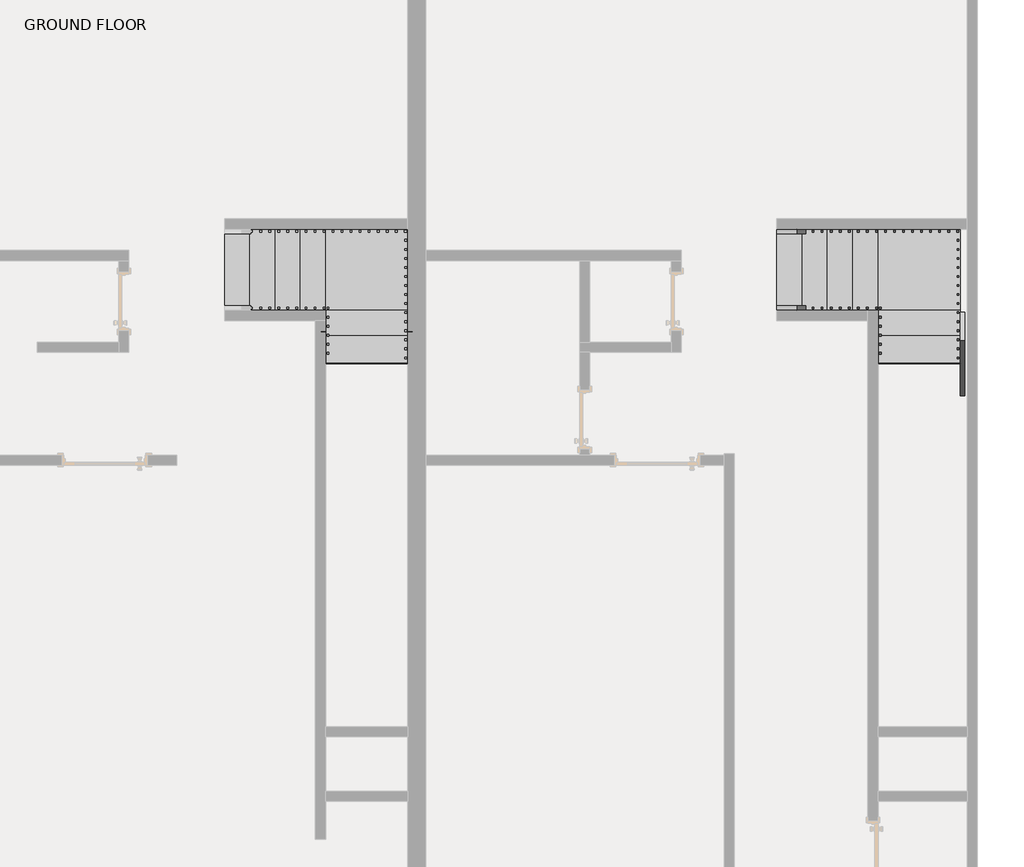
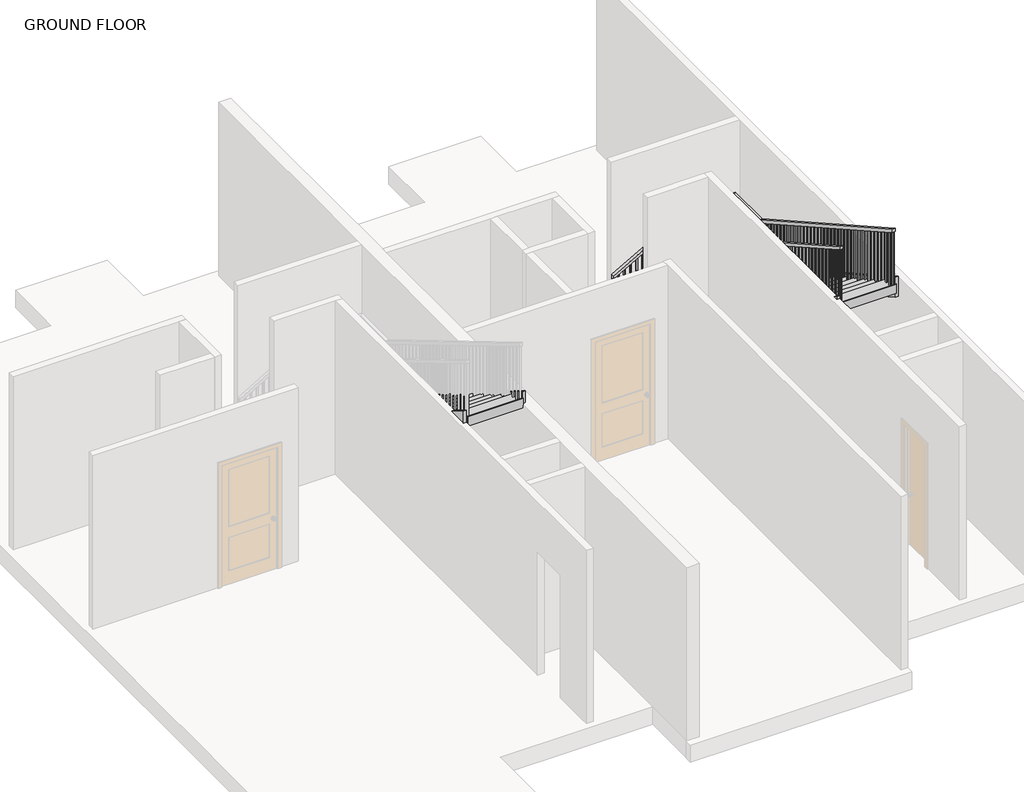
# One storey, part 4 of 4: 8 members, 2 railings, 2 stair flights.
"""IFC4 building model written with IfcOpenShell, lengths in millimetres."""

from ifc_helpers import new_model, si_unit, frame, origin, place, context, project, spatial, polyline, outline, extrude, faceted_brep, transform, mapped, element, save
from components import stair_flight_9587ce78, stair_flight_92322d8c

model = new_model("IFC4")

# Units and contexts
model_context = context("Model", 3, world=origin())
ifc_project = project(units=[si_unit("LENGTHUNIT", "METRE", prefix="MILLI")], contexts=[model_context])

# Site, building, storey
site = spatial("IfcSite", under=ifc_project)
building = spatial("IfcBuilding", under=site)
storey = spatial("IfcBuildingStorey", under=building, Name="GROUND FLOOR", Elevation=304.8)

# Members
placement = place(None, origin())
element("IfcMember", 1, ObjectType="Stringer - 2\" Width", at=placement, inside=storey, context=model_context, shape_type="SweptSolid", body=[
    extrude(outline(polyline([(516.0200704, -14204.9595293), (304.8, -14204.9595293), (304.8, -13964.03282), (818.2858896, -13102.7637874), (818.2858896, -13697.9695712), (516.0200704, -14204.9595293)])), frame((0.0, 4044.5909199, 0.0), z_axis=(0.0, 1.0, 0.0), x_axis=(0.0, 0.0, 1.0)), (0.0, 0.0, 1.0), 50.8),
])
element("IfcMember", 2, ObjectType="Stringer - 2\" Width", at=placement, inside=storey, context=model_context, shape_type="SweptSolid", body=[
    extrude(outline(polyline([(2488.0796213, 1390.0849918), (-567.9697052, 3209.1936945), (-567.9697052, 3563.90557), (3083.9851801, 1390.0849918), (2488.0796213, 1390.0849918)])), frame((-12143.6860997, 0.0, 0.0), z_axis=(1.0, 0.0, 0.0), x_axis=(0.0, 1.0, 0.0)), (0.0, 0.0, 1.0), 50.8),
])
element("IfcMember", 3, ObjectType="Stringer - 2\" Width", at=placement, inside=storey, context=model_context, shape_type="SweptSolid", body=[
    extrude(outline(polyline([(516.0200704, -14204.9595293), (304.8, -14204.9595293), (304.8, -13964.03282), (808.1881543, -13119.7007021), (1163.0479714, -13119.7007021), (516.0200704, -14204.9595293)])), frame((0.0, 3079.3909199, 0.0), z_axis=(0.0, 1.0, 0.0), x_axis=(0.0, 0.0, 1.0)), (0.0, 0.0, 1.0), 50.8),
])
element("IfcMember", 4, ObjectType="Stringer - 2\" Width", at=placement, inside=storey, context=model_context, shape_type="SweptSolid", body=[
    extrude(outline(polyline([(3130.1909199, 1362.5810956), (3130.1909199, 1007.8692202), (-567.9697052, 3209.1936945), (-567.9697052, 3563.90557), (3130.1909199, 1362.5810956)])), frame((-13119.7007021, 0.0, 0.0), z_axis=(1.0, 0.0, 0.0), x_axis=(0.0, 1.0, 0.0)), (0.0, 0.0, 1.0), 50.8),
])
element("IfcMember", 5, ObjectType="Stringer - 2\" Width", at=placement, inside=storey, context=model_context, shape_type="SweptSolid", body=[
    extrude(outline(polyline([(513.2142827, -7996.544927), (304.8, -7996.544927), (304.8, -7745.7665395), (799.5757743, -6869.775142), (799.5757743, -7489.5471791), (513.2142827, -7996.544927)])), frame((0.0, 4044.5909199, 0.0), z_axis=(0.0, 1.0, 0.0), x_axis=(0.0, 0.0, 1.0)), (0.0, 0.0, 1.0), 50.8),
])
element("IfcMember", 6, ObjectType="Stringer - 2\" Width", at=placement, inside=storey, context=model_context, shape_type="SweptSolid", body=[
    extrude(outline(polyline([(2488.0775681, 1327.4003232), (-567.9697052, 3050.7653048), (-567.9697052, 3400.6891557), (3108.5983757, 1327.4003232), (2488.0775681, 1327.4003232)])), frame((-5935.2714974, 0.0, 0.0), z_axis=(1.0, 0.0, 0.0), x_axis=(0.0, 1.0, 0.0)), (0.0, 0.0, 1.0), 50.8),
])
element("IfcMember", 7, ObjectType="Stringer - 2\" Width", at=placement, inside=storey, context=model_context, shape_type="SweptSolid", body=[
    extrude(outline(polyline([(513.2142827, -7996.544927), (304.8, -7996.544927), (304.8, -7745.7665395), (776.1296351, -6911.2860997), (1126.1880836, -6911.2860997), (513.2142827, -7996.544927)])), frame((0.0, 3079.3909199, 0.0), z_axis=(0.0, 1.0, 0.0), x_axis=(0.0, 0.0, 1.0)), (0.0, 0.0, 1.0), 50.8),
])
element("IfcMember", 8, ObjectType="Stringer - 2\" Width", at=placement, inside=storey, context=model_context, shape_type="SweptSolid", body=[
    extrude(outline(polyline([(3130.1909199, 1315.2238642), (3130.1909199, 965.3000133), (-567.9697052, 3050.7653048), (-567.9697052, 3400.6891557), (3130.1909199, 1315.2238642)])), frame((-6911.2860997, 0.0, 0.0), z_axis=(1.0, 0.0, 0.0), x_axis=(0.0, 1.0, 0.0)), (0.0, 0.0, 1.0), 50.8),
])

# Railings
element("IfcRailing", 9, ObjectType="Handrail - Rectangular", at=placement, inside=storey, context=model_context, shape_type="SolidModel", body=[
    faceted_brep([(-7996.544927, 3180.9909199, 1379.6210526), (-7996.544927, 3180.9909199, 1321.2775897), (-7996.544927, 3130.1909199, 1321.2775897), (-7996.544927, 3130.1909199, 1379.6210526), (-6936.6860997, 3180.9909199, 1978.2649419), (-6885.8860997, 3180.9909199, 1948.6150265), (-6885.8860997, 3130.1909199, 1948.6150265), (-6936.6860997, 3130.1909199, 1978.2649419), (-6936.6860997, 3180.9909199, 2224.6971629), (-6885.8860997, 3180.9909199, 2173.8971629), (-6885.8860997, 3130.1909199, 2173.8971629), (-6936.6860997, 3130.1909199, 2224.6971629), (-6809.6860997, 3180.9909199, 2224.6971629), (-6809.6860997, 3180.9909199, 2173.8971629), (-6860.4860997, 3130.1909199, 2173.8971629), (-6860.4860997, 3130.1909199, 2224.6971629), (-6809.6860997, 3053.9909199, 2224.6971629), (-6809.6860997, 3040.6545009, 2173.8971629), (-6860.4860997, 3040.6545009, 2173.8971629), (-6860.4860997, 3053.9909199, 2224.6971629), (-6809.6860997, -567.9697052, 4267.2), (-6860.4860997, -567.9697052, 4267.2), (-6860.4860997, -567.9697052, 4208.8793016), (-6809.6860997, -567.9697052, 4208.8793016)], [[[0, 1, 2, 3]], [[1, 0, 4, 5]], [[2, 1, 5, 6]], [[3, 2, 6, 7]], [[0, 3, 7, 4]], [[5, 4, 8, 9]], [[6, 5, 9, 10]], [[7, 6, 10, 11]], [[4, 7, 11, 8]], [[9, 8, 12, 13]], [[10, 9, 13, 14]], [[11, 10, 14, 15]], [[8, 11, 15, 12]], [[13, 12, 16, 17]], [[14, 13, 17, 18]], [[15, 14, 18, 19]], [[12, 15, 19, 16]], [[20, 21, 22, 23]], [[17, 16, 20, 23]], [[18, 17, 23, 22]], [[19, 18, 22, 21]], [[16, 19, 21, 20]]]),
    extrude(outline(polyline([(-511.5340801, 4177.0195862), (-492.4840801, 4166.2768744), (-492.4840801, 3192.3789474), (-511.5340801, 3192.3789474), (-511.5340801, 4177.0195862)])), frame((-6844.6110997, 0.0, 0.0), z_axis=(1.0, 0.0, 0.0), x_axis=(0.0, 1.0, 0.0)), (0.0, 0.0, 1.0), 19.05),
    extrude(outline(polyline([(-409.9340801, 4119.7251234), (-390.8840801, 4108.9824116), (-390.8840801, 3192.3789474), (-409.9340801, 3192.3789474), (-409.9340801, 4119.7251234)])), frame((-6844.6110997, 0.0, 0.0), z_axis=(1.0, 0.0, 0.0), x_axis=(0.0, 1.0, 0.0)), (0.0, 0.0, 1.0), 19.05),
    extrude(outline(polyline([(-308.3340801, 4062.4306606), (-289.2840801, 4051.6879488), (-289.2840801, 3192.3789474), (-308.3340801, 3192.3789474), (-308.3340801, 4062.4306606)])), frame((-6844.6110997, 0.0, 0.0), z_axis=(1.0, 0.0, 0.0), x_axis=(0.0, 1.0, 0.0)), (0.0, 0.0, 1.0), 19.05),
    extrude(outline(polyline([(-206.7340801, 4005.1361978), (-187.6840801, 3994.393486), (-187.6840801, 3031.9578947), (-206.7340801, 3031.9578947), (-206.7340801, 4005.1361978)])), frame((-6844.6110997, 0.0, 0.0), z_axis=(1.0, 0.0, 0.0), x_axis=(0.0, 1.0, 0.0)), (0.0, 0.0, 1.0), 19.05),
    extrude(outline(polyline([(-105.1340801, 3947.841735), (-86.0840801, 3937.0990232), (-86.0840801, 3031.9578947), (-105.1340801, 3031.9578947), (-105.1340801, 3947.841735)])), frame((-6844.6110997, 0.0, 0.0), z_axis=(1.0, 0.0, 0.0), x_axis=(0.0, 1.0, 0.0)), (0.0, 0.0, 1.0), 19.05),
    extrude(outline(polyline([(-3.5340801, 3890.5472722), (15.5159199, 3879.8045604), (15.5159199, 2871.5368421), (-3.5340801, 2871.5368421), (-3.5340801, 3890.5472722)])), frame((-6844.6110997, 0.0, 0.0), z_axis=(1.0, 0.0, 0.0), x_axis=(0.0, 1.0, 0.0)), (0.0, 0.0, 1.0), 19.05),
    extrude(outline(polyline([(98.0659199, 3833.2528094), (117.1159199, 3822.5100977), (117.1159199, 2871.5368421), (98.0659199, 2871.5368421), (98.0659199, 3833.2528094)])), frame((-6844.6110997, 0.0, 0.0), z_axis=(1.0, 0.0, 0.0), x_axis=(0.0, 1.0, 0.0)), (0.0, 0.0, 1.0), 19.05),
    extrude(outline(polyline([(199.6659199, 3775.9583466), (218.7159199, 3765.2156349), (218.7159199, 2871.5368421), (199.6659199, 2871.5368421), (199.6659199, 3775.9583466)])), frame((-6844.6110997, 0.0, 0.0), z_axis=(1.0, 0.0, 0.0), x_axis=(0.0, 1.0, 0.0)), (0.0, 0.0, 1.0), 19.05),
    extrude(outline(polyline([(301.2659199, 3718.6810997), (320.3159199, 3707.938388), (320.3159199, 2711.1157895), (301.2659199, 2711.1157895), (301.2659199, 3718.6810997)])), frame((-6844.6110997, 0.0, 0.0), z_axis=(1.0, 0.0, 0.0), x_axis=(0.0, 1.0, 0.0)), (0.0, 0.0, 1.0), 19.05),
    extrude(outline(polyline([(402.8659199, 3661.3866369), (421.9159199, 3650.6439252), (421.9159199, 2711.1157895), (402.8659199, 2711.1157895), (402.8659199, 3661.3866369)])), frame((-6844.6110997, 0.0, 0.0), z_axis=(1.0, 0.0, 0.0), x_axis=(0.0, 1.0, 0.0)), (0.0, 0.0, 1.0), 19.05),
    extrude(outline(polyline([(504.4659199, 3604.0921741), (523.5159199, 3593.3494624), (523.5159199, 2711.1157895), (504.4659199, 2711.1157895), (504.4659199, 3604.0921741)])), frame((-6844.6110997, 0.0, 0.0), z_axis=(1.0, 0.0, 0.0), x_axis=(0.0, 1.0, 0.0)), (0.0, 0.0, 1.0), 19.05),
    extrude(outline(polyline([(606.0659199, 3546.7977114), (625.1159199, 3536.0549996), (625.1159199, 2550.6947368), (606.0659199, 2550.6947368), (606.0659199, 3546.7977114)])), frame((-6844.6110997, 0.0, 0.0), z_axis=(1.0, 0.0, 0.0), x_axis=(0.0, 1.0, 0.0)), (0.0, 0.0, 1.0), 19.05),
    extrude(outline(polyline([(707.6659199, 3489.5032486), (726.7159199, 3478.7605368), (726.7159199, 2550.6947368), (707.6659199, 2550.6947368), (707.6659199, 3489.5032486)])), frame((-6844.6110997, 0.0, 0.0), z_axis=(1.0, 0.0, 0.0), x_axis=(0.0, 1.0, 0.0)), (0.0, 0.0, 1.0), 19.05),
    extrude(outline(polyline([(809.2659199, 3432.2087858), (828.3159199, 3421.466074), (828.3159199, 2550.6947368), (809.2659199, 2550.6947368), (809.2659199, 3432.2087858)])), frame((-6844.6110997, 0.0, 0.0), z_axis=(1.0, 0.0, 0.0), x_axis=(0.0, 1.0, 0.0)), (0.0, 0.0, 1.0), 19.05),
    extrude(outline(polyline([(910.8659199, 3374.914323), (929.9159199, 3364.1716112), (929.9159199, 2390.2736842), (910.8659199, 2390.2736842), (910.8659199, 3374.914323)])), frame((-6844.6110997, 0.0, 0.0), z_axis=(1.0, 0.0, 0.0), x_axis=(0.0, 1.0, 0.0)), (0.0, 0.0, 1.0), 19.05),
    extrude(outline(polyline([(1012.4659199, 3317.6198602), (1031.5159199, 3306.8771484), (1031.5159199, 2390.2736842), (1012.4659199, 2390.2736842), (1012.4659199, 3317.6198602)])), frame((-6844.6110997, 0.0, 0.0), z_axis=(1.0, 0.0, 0.0), x_axis=(0.0, 1.0, 0.0)), (0.0, 0.0, 1.0), 19.05),
    extrude(outline(polyline([(1114.0659199, 3260.3253974), (1133.1159199, 3249.5826857), (1133.1159199, 2390.2736842), (1114.0659199, 2390.2736842), (1114.0659199, 3260.3253974)])), frame((-6844.6110997, 0.0, 0.0), z_axis=(1.0, 0.0, 0.0), x_axis=(0.0, 1.0, 0.0)), (0.0, 0.0, 1.0), 19.05),
    extrude(outline(polyline([(1215.6659199, 3203.0309346), (1234.7159199, 3192.2882229), (1234.7159199, 2229.8526316), (1215.6659199, 2229.8526316), (1215.6659199, 3203.0309346)])), frame((-6844.6110997, 0.0, 0.0), z_axis=(1.0, 0.0, 0.0), x_axis=(0.0, 1.0, 0.0)), (0.0, 0.0, 1.0), 19.05),
    extrude(outline(polyline([(1317.2659199, 3145.7364718), (1336.3159199, 3134.9937601), (1336.3159199, 2229.8526316), (1317.2659199, 2229.8526316), (1317.2659199, 3145.7364718)])), frame((-6844.6110997, 0.0, 0.0), z_axis=(1.0, 0.0, 0.0), x_axis=(0.0, 1.0, 0.0)), (0.0, 0.0, 1.0), 19.05),
    extrude(outline(polyline([(1418.8659199, 3088.4420091), (1437.9159199, 3077.6992973), (1437.9159199, 2069.4315789), (1418.8659199, 2069.4315789), (1418.8659199, 3088.4420091)])), frame((-6844.6110997, 0.0, 0.0), z_axis=(1.0, 0.0, 0.0), x_axis=(0.0, 1.0, 0.0)), (0.0, 0.0, 1.0), 19.05),
    extrude(outline(polyline([(1520.4659199, 3031.1475463), (1539.5159199, 3020.4048345), (1539.5159199, 2069.4315789), (1520.4659199, 2069.4315789), (1520.4659199, 3031.1475463)])), frame((-6844.6110997, 0.0, 0.0), z_axis=(1.0, 0.0, 0.0), x_axis=(0.0, 1.0, 0.0)), (0.0, 0.0, 1.0), 19.05),
    extrude(outline(polyline([(1622.0659199, 2973.8530835), (1641.1159199, 2963.1103717), (1641.1159199, 2069.4315789), (1622.0659199, 2069.4315789), (1622.0659199, 2973.8530835)])), frame((-6844.6110997, 0.0, 0.0), z_axis=(1.0, 0.0, 0.0), x_axis=(0.0, 1.0, 0.0)), (0.0, 0.0, 1.0), 19.05),
    extrude(outline(polyline([(1723.6659199, 2916.5758366), (1742.7159199, 2905.8331248), (1742.7159199, 1909.0105263), (1723.6659199, 1909.0105263), (1723.6659199, 2916.5758366)])), frame((-6844.6110997, 0.0, 0.0), z_axis=(1.0, 0.0, 0.0), x_axis=(0.0, 1.0, 0.0)), (0.0, 0.0, 1.0), 19.05),
    extrude(outline(polyline([(1825.2659199, 2859.2813738), (1844.3159199, 2848.538662), (1844.3159199, 1909.0105263), (1825.2659199, 1909.0105263), (1825.2659199, 2859.2813738)])), frame((-6844.6110997, 0.0, 0.0), z_axis=(1.0, 0.0, 0.0), x_axis=(0.0, 1.0, 0.0)), (0.0, 0.0, 1.0), 19.05),
    extrude(outline(polyline([(1926.8659199, 2801.986911), (1945.9159199, 2791.2441992), (1945.9159199, 1909.0105263), (1926.8659199, 1909.0105263), (1926.8659199, 2801.986911)])), frame((-6844.6110997, 0.0, 0.0), z_axis=(1.0, 0.0, 0.0), x_axis=(0.0, 1.0, 0.0)), (0.0, 0.0, 1.0), 19.05),
    extrude(outline(polyline([(2028.4659199, 2744.6924482), (2047.5159199, 2733.9497364), (2047.5159199, 1748.5894737), (2028.4659199, 1748.5894737), (2028.4659199, 2744.6924482)])), frame((-6844.6110997, 0.0, 0.0), z_axis=(1.0, 0.0, 0.0), x_axis=(0.0, 1.0, 0.0)), (0.0, 0.0, 1.0), 19.05),
    extrude(outline(polyline([(2130.0659199, 2687.3979854), (2149.1159199, 2676.6552736), (2149.1159199, 1748.5894737), (2130.0659199, 1748.5894737), (2130.0659199, 2687.3979854)])), frame((-6844.6110997, 0.0, 0.0), z_axis=(1.0, 0.0, 0.0), x_axis=(0.0, 1.0, 0.0)), (0.0, 0.0, 1.0), 19.05),
    extrude(outline(polyline([(2231.6659199, 2630.1035226), (2250.7159199, 2619.3608109), (2250.7159199, 1748.5894737), (2231.6659199, 1748.5894737), (2231.6659199, 2630.1035226)])), frame((-6844.6110997, 0.0, 0.0), z_axis=(1.0, 0.0, 0.0), x_axis=(0.0, 1.0, 0.0)), (0.0, 0.0, 1.0), 19.05),
    extrude(outline(polyline([(2333.2659199, 2572.8090598), (2352.3159199, 2562.0663481), (2352.3159199, 1588.1684211), (2333.2659199, 1588.1684211), (2333.2659199, 2572.8090598)])), frame((-6844.6110997, 0.0, 0.0), z_axis=(1.0, 0.0, 0.0), x_axis=(0.0, 1.0, 0.0)), (0.0, 0.0, 1.0), 19.05),
    extrude(outline(polyline([(2434.8659199, 2515.5145971), (2453.9159199, 2504.7718853), (2453.9159199, 1588.1684211), (2434.8659199, 1588.1684211), (2434.8659199, 2515.5145971)])), frame((-6844.6110997, 0.0, 0.0), z_axis=(1.0, 0.0, 0.0), x_axis=(0.0, 1.0, 0.0)), (0.0, 0.0, 1.0), 19.05),
    extrude(outline(polyline([(2536.4659199, 2458.2201343), (2555.5159199, 2447.4774225), (2555.5159199, 1588.1684211), (2536.4659199, 1588.1684211), (2536.4659199, 2458.2201343)])), frame((-6844.6110997, 0.0, 0.0), z_axis=(1.0, 0.0, 0.0), x_axis=(0.0, 1.0, 0.0)), (0.0, 0.0, 1.0), 19.05),
    extrude(outline(polyline([(2638.0659199, 2400.9256715), (2657.1159199, 2390.1829597), (2657.1159199, 1427.7473684), (2638.0659199, 1427.7473684), (2638.0659199, 2400.9256715)])), frame((-6844.6110997, 0.0, 0.0), z_axis=(1.0, 0.0, 0.0), x_axis=(0.0, 1.0, 0.0)), (0.0, 0.0, 1.0), 19.05),
    extrude(outline(polyline([(2739.6659199, 2343.6312087), (2758.7159199, 2332.8884969), (2758.7159199, 1427.7473684), (2739.6659199, 1427.7473684), (2739.6659199, 2343.6312087)])), frame((-6844.6110997, 0.0, 0.0), z_axis=(1.0, 0.0, 0.0), x_axis=(0.0, 1.0, 0.0)), (0.0, 0.0, 1.0), 19.05),
    extrude(outline(polyline([(2841.2659199, 2286.3367459), (2860.3159199, 2275.5940341), (2860.3159199, 1267.3263158), (2841.2659199, 1267.3263158), (2841.2659199, 2286.3367459)])), frame((-6844.6110997, 0.0, 0.0), z_axis=(1.0, 0.0, 0.0), x_axis=(0.0, 1.0, 0.0)), (0.0, 0.0, 1.0), 19.05),
    extrude(outline(polyline([(2942.8659199, 2229.0422831), (2961.9159199, 2218.2995713), (2961.9159199, 1267.3263158), (2942.8659199, 1267.3263158), (2942.8659199, 2229.0422831)])), frame((-6844.6110997, 0.0, 0.0), z_axis=(1.0, 0.0, 0.0), x_axis=(0.0, 1.0, 0.0)), (0.0, 0.0, 1.0), 19.05),
    extrude(outline(polyline([(3044.4659199, 2171.7478203), (3063.5159199, 2161.0051086), (3063.5159199, 1267.3263158), (3044.4659199, 1267.3263158), (3044.4659199, 2171.7478203)])), frame((-6844.6110997, 0.0, 0.0), z_axis=(1.0, 0.0, 0.0), x_axis=(0.0, 1.0, 0.0)), (0.0, 0.0, 1.0), 19.05),
    extrude(outline(polyline([(-6888.469927, 3146.0659199), (-6888.469927, 3165.1159199), (-6869.419927, 3165.1159199), (-6869.419927, 3146.0659199), (-6888.469927, 3146.0659199)])), frame((0.0, 0.0, 946.4842105), z_axis=(0.0, 0.0, 1.0), x_axis=(1.0, 0.0, 0.0)), (0.0, 0.0, 1.0), 1227.4129524),
    extrude(outline(polyline([(1900.5285794, -6971.019927), (1889.7684991, -6990.069927), (946.4842105, -6990.069927), (946.4842105, -6971.019927), (1900.5285794, -6971.019927)])), frame((0.0, 3146.0659199, 0.0), z_axis=(0.0, 1.0, 0.0), x_axis=(0.0, 0.0, 1.0)), (0.0, 0.0, 1.0), 19.05),
    extrude(outline(polyline([(1843.1414844, -7072.619927), (1832.3814041, -7091.669927), (946.4842105, -7091.669927), (946.4842105, -7072.619927), (1843.1414844, -7072.619927)])), frame((0.0, 3146.0659199, 0.0), z_axis=(0.0, 1.0, 0.0), x_axis=(0.0, 0.0, 1.0)), (0.0, 0.0, 1.0), 19.05),
    extrude(outline(polyline([(1785.7543895, -7174.219927), (1774.9943092, -7193.269927), (786.0631579, -7193.269927), (786.0631579, -7174.219927), (1785.7543895, -7174.219927)])), frame((0.0, 3146.0659199, 0.0), z_axis=(0.0, 1.0, 0.0), x_axis=(0.0, 0.0, 1.0)), (0.0, 0.0, 1.0), 19.05),
    extrude(outline(polyline([(1728.3672945, -7275.819927), (1717.6072142, -7294.869927), (786.0631579, -7294.869927), (786.0631579, -7275.819927), (1728.3672945, -7275.819927)])), frame((0.0, 3146.0659199, 0.0), z_axis=(0.0, 1.0, 0.0), x_axis=(0.0, 0.0, 1.0)), (0.0, 0.0, 1.0), 19.05),
    extrude(outline(polyline([(1670.9801996, -7377.419927), (1660.2201193, -7396.469927), (786.0631579, -7396.469927), (786.0631579, -7377.419927), (1670.9801996, -7377.419927)])), frame((0.0, 3146.0659199, 0.0), z_axis=(0.0, 1.0, 0.0), x_axis=(0.0, 0.0, 1.0)), (0.0, 0.0, 1.0), 19.05),
    extrude(outline(polyline([(1613.5931046, -7479.019927), (1602.8330243, -7498.069927), (625.6421053, -7498.069927), (625.6421053, -7479.019927), (1613.5931046, -7479.019927)])), frame((0.0, 3146.0659199, 0.0), z_axis=(0.0, 1.0, 0.0), x_axis=(0.0, 0.0, 1.0)), (0.0, 0.0, 1.0), 19.05),
    extrude(outline(polyline([(1556.2060097, -7580.619927), (1545.4459294, -7599.669927), (625.6421053, -7599.669927), (625.6421053, -7580.619927), (1556.2060097, -7580.619927)])), frame((0.0, 3146.0659199, 0.0), z_axis=(0.0, 1.0, 0.0), x_axis=(0.0, 0.0, 1.0)), (0.0, 0.0, 1.0), 19.05),
    extrude(outline(polyline([(1498.8189147, -7682.219927), (1488.0588344, -7701.269927), (625.6421053, -7701.269927), (625.6421053, -7682.219927), (1498.8189147, -7682.219927)])), frame((0.0, 3146.0659199, 0.0), z_axis=(0.0, 1.0, 0.0), x_axis=(0.0, 0.0, 1.0)), (0.0, 0.0, 1.0), 19.05),
    extrude(outline(polyline([(1441.4318198, -7783.819927), (1430.6717395, -7802.869927), (465.2210526, -7802.869927), (465.2210526, -7783.819927), (1441.4318198, -7783.819927)])), frame((0.0, 3146.0659199, 0.0), z_axis=(0.0, 1.0, 0.0), x_axis=(0.0, 0.0, 1.0)), (0.0, 0.0, 1.0), 19.05),
    extrude(outline(polyline([(1384.0447248, -7885.419927), (1373.2846445, -7904.469927), (465.2210526, -7904.469927), (465.2210526, -7885.419927), (1384.0447248, -7885.419927)])), frame((0.0, 3146.0659199, 0.0), z_axis=(0.0, 1.0, 0.0), x_axis=(0.0, 0.0, 1.0)), (0.0, 0.0, 1.0), 19.05),
    extrude(outline(polyline([(-6844.6110997, 3146.0659199), (-6844.6110997, 3165.1159199), (-6825.5610997, 3165.1159199), (-6825.5610997, 3146.0659199), (-6844.6110997, 3146.0659199)])), frame((0.0, 0.0, 1106.9052632), z_axis=(0.0, 0.0, 1.0), x_axis=(1.0, 0.0, 0.0)), (0.0, 0.0, 1.0), 1066.9918997),
    extrude(outline(polyline([(-567.9697052, 4208.8793016), (-548.9197052, 4198.1365898), (-548.9197052, 3192.3789474), (-567.9697052, 3192.3789474), (-567.9697052, 4208.8793016)])), frame((-6844.6110997, 0.0, 0.0), z_axis=(1.0, 0.0, 0.0), x_axis=(0.0, 1.0, 0.0)), (0.0, 0.0, 1.0), 19.05),
    extrude(outline(polyline([(1332.03767, -7977.494927), (1321.2775897, -7996.544927), (465.2210526, -7996.544927), (465.2210526, -7977.494927), (1332.03767, -7977.494927)])), frame((0.0, 3146.0659199, 0.0), z_axis=(0.0, 1.0, 0.0), x_axis=(0.0, 0.0, 1.0)), (0.0, 0.0, 1.0), 19.05),
])
element("IfcRailing", 10, ObjectType="Handrail - Rectangular", at=placement, inside=storey, context=model_context, shape_type="SolidModel", body=[
    faceted_brep([(-7996.544927, 4044.5909199, 1379.6210526), (-7996.544927, 4044.5909199, 1321.2775897), (-7996.544927, 3993.7909199, 1321.2775897), (-7996.544927, 3993.7909199, 1379.6210526), (-6712.3539494, 4044.5909199, 2104.9752806), (-6698.9987546, 4044.5909199, 2054.1752806), (-6698.9987546, 3993.7909199, 2054.1752806), (-6712.3539494, 3993.7909199, 2104.9752806), (-5935.2714974, 4044.5909199, 2104.9752806), (-5935.2714974, 4044.5909199, 2054.1752806), (-5986.0714974, 3993.7909199, 2054.1752806), (-5986.0714974, 3993.7909199, 2104.9752806), (-5935.2714974, 3266.2931677, 2104.9752806), (-5935.2714974, 3252.9567487, 2054.1752806), (-5986.0714974, 3252.9567487, 2054.1752806), (-5986.0714974, 3266.2931677, 2104.9752806), (-5935.2714974, -567.9697052, 4267.2), (-5986.0714974, -567.9697052, 4267.2), (-5986.0714974, -567.9697052, 4208.8793016), (-5935.2714974, -567.9697052, 4208.8793016)], [[[0, 1, 2, 3]], [[1, 0, 4, 5]], [[2, 1, 5, 6]], [[3, 2, 6, 7]], [[0, 3, 7, 4]], [[5, 4, 8, 9]], [[6, 5, 9, 10]], [[7, 6, 10, 11]], [[4, 7, 11, 8]], [[9, 8, 12, 13]], [[10, 9, 13, 14]], [[11, 10, 14, 15]], [[8, 11, 15, 12]], [[16, 17, 18, 19]], [[13, 12, 16, 19]], [[14, 13, 19, 18]], [[15, 14, 18, 17]], [[12, 15, 17, 16]]]),
    extrude(outline(polyline([(-543.2840801, 4194.9241058), (-543.2840801, 3192.3789474), (-562.3340801, 3192.3789474), (-562.3340801, 4205.6668176), (-543.2840801, 4194.9241058)])), frame((-5970.1964974, 0.0, 0.0), z_axis=(1.0, 0.0, 0.0), x_axis=(0.0, 1.0, 0.0)), (0.0, 0.0, 1.0), 19.05),
    extrude(outline(polyline([(-441.6840801, 4137.629643), (-441.6840801, 3192.3789474), (-460.7340801, 3192.3789474), (-460.7340801, 4148.3723548), (-441.6840801, 4137.629643)])), frame((-5970.1964974, 0.0, 0.0), z_axis=(1.0, 0.0, 0.0), x_axis=(0.0, 1.0, 0.0)), (0.0, 0.0, 1.0), 19.05),
    extrude(outline(polyline([(-340.0840801, 4080.3351802), (-340.0840801, 3192.3789474), (-359.1340801, 3192.3789474), (-359.1340801, 4091.077892), (-340.0840801, 4080.3351802)])), frame((-5970.1964974, 0.0, 0.0), z_axis=(1.0, 0.0, 0.0), x_axis=(0.0, 1.0, 0.0)), (0.0, 0.0, 1.0), 19.05),
    extrude(outline(polyline([(-238.4840801, 4023.0407174), (-238.4840801, 3031.9578947), (-257.5340801, 3031.9578947), (-257.5340801, 4033.7834292), (-238.4840801, 4023.0407174)])), frame((-5970.1964974, 0.0, 0.0), z_axis=(1.0, 0.0, 0.0), x_axis=(0.0, 1.0, 0.0)), (0.0, 0.0, 1.0), 19.05),
    extrude(outline(polyline([(-136.8840801, 3965.7462546), (-136.8840801, 3031.9578947), (-155.9340801, 3031.9578947), (-155.9340801, 3976.4889664), (-136.8840801, 3965.7462546)])), frame((-5970.1964974, 0.0, 0.0), z_axis=(1.0, 0.0, 0.0), x_axis=(0.0, 1.0, 0.0)), (0.0, 0.0, 1.0), 19.05),
    extrude(outline(polyline([(-35.2840801, 3908.4517918), (-35.2840801, 3031.9578947), (-54.3340801, 3031.9578947), (-54.3340801, 3919.1945036), (-35.2840801, 3908.4517918)])), frame((-5970.1964974, 0.0, 0.0), z_axis=(1.0, 0.0, 0.0), x_axis=(0.0, 1.0, 0.0)), (0.0, 0.0, 1.0), 19.05),
    extrude(outline(polyline([(66.3159199, 3851.1573291), (66.3159199, 2871.5368421), (47.2659199, 2871.5368421), (47.2659199, 3861.9000408), (66.3159199, 3851.1573291)])), frame((-5970.1964974, 0.0, 0.0), z_axis=(1.0, 0.0, 0.0), x_axis=(0.0, 1.0, 0.0)), (0.0, 0.0, 1.0), 19.05),
    extrude(outline(polyline([(167.9159199, 3793.8628663), (167.9159199, 2871.5368421), (148.8659199, 2871.5368421), (148.8659199, 3804.605578), (167.9159199, 3793.8628663)])), frame((-5970.1964974, 0.0, 0.0), z_axis=(1.0, 0.0, 0.0), x_axis=(0.0, 1.0, 0.0)), (0.0, 0.0, 1.0), 19.05),
    extrude(outline(polyline([(269.5159199, 3736.5684035), (269.5159199, 2871.5368421), (250.4659199, 2871.5368421), (250.4659199, 3747.3111152), (269.5159199, 3736.5684035)])), frame((-5970.1964974, 0.0, 0.0), z_axis=(1.0, 0.0, 0.0), x_axis=(0.0, 1.0, 0.0)), (0.0, 0.0, 1.0), 19.05),
    extrude(outline(polyline([(371.1159199, 3679.2739407), (371.1159199, 2711.1157895), (352.0659199, 2711.1157895), (352.0659199, 3690.0166525), (371.1159199, 3679.2739407)])), frame((-5970.1964974, 0.0, 0.0), z_axis=(1.0, 0.0, 0.0), x_axis=(0.0, 1.0, 0.0)), (0.0, 0.0, 1.0), 19.05),
    extrude(outline(polyline([(472.7159199, 3621.9966938), (472.7159199, 2711.1157895), (453.6659199, 2711.1157895), (453.6659199, 3632.7394055), (472.7159199, 3621.9966938)])), frame((-5970.1964974, 0.0, 0.0), z_axis=(1.0, 0.0, 0.0), x_axis=(0.0, 1.0, 0.0)), (0.0, 0.0, 1.0), 19.05),
    extrude(outline(polyline([(574.3159199, 3564.702231), (574.3159199, 2711.1157895), (555.2659199, 2711.1157895), (555.2659199, 3575.4449428), (574.3159199, 3564.702231)])), frame((-5970.1964974, 0.0, 0.0), z_axis=(1.0, 0.0, 0.0), x_axis=(0.0, 1.0, 0.0)), (0.0, 0.0, 1.0), 19.05),
    extrude(outline(polyline([(675.9159199, 3507.4077682), (675.9159199, 2550.6947368), (656.8659199, 2550.6947368), (656.8659199, 3518.15048), (675.9159199, 3507.4077682)])), frame((-5970.1964974, 0.0, 0.0), z_axis=(1.0, 0.0, 0.0), x_axis=(0.0, 1.0, 0.0)), (0.0, 0.0, 1.0), 19.05),
    extrude(outline(polyline([(777.5159199, 3450.1133054), (777.5159199, 2550.6947368), (758.4659199, 2550.6947368), (758.4659199, 3460.8560172), (777.5159199, 3450.1133054)])), frame((-5970.1964974, 0.0, 0.0), z_axis=(1.0, 0.0, 0.0), x_axis=(0.0, 1.0, 0.0)), (0.0, 0.0, 1.0), 19.05),
    extrude(outline(polyline([(879.1159199, 3392.8188426), (879.1159199, 2390.2736842), (860.0659199, 2390.2736842), (860.0659199, 3403.5615544), (879.1159199, 3392.8188426)])), frame((-5970.1964974, 0.0, 0.0), z_axis=(1.0, 0.0, 0.0), x_axis=(0.0, 1.0, 0.0)), (0.0, 0.0, 1.0), 19.05),
    extrude(outline(polyline([(980.7159199, 3335.5243798), (980.7159199, 2390.2736842), (961.6659199, 2390.2736842), (961.6659199, 3346.2670916), (980.7159199, 3335.5243798)])), frame((-5970.1964974, 0.0, 0.0), z_axis=(1.0, 0.0, 0.0), x_axis=(0.0, 1.0, 0.0)), (0.0, 0.0, 1.0), 19.05),
    extrude(outline(polyline([(1082.3159199, 3278.229917), (1082.3159199, 2390.2736842), (1063.2659199, 2390.2736842), (1063.2659199, 3288.9726288), (1082.3159199, 3278.229917)])), frame((-5970.1964974, 0.0, 0.0), z_axis=(1.0, 0.0, 0.0), x_axis=(0.0, 1.0, 0.0)), (0.0, 0.0, 1.0), 19.05),
    extrude(outline(polyline([(1183.9159199, 3220.9354543), (1183.9159199, 2229.8526316), (1164.8659199, 2229.8526316), (1164.8659199, 3231.678166), (1183.9159199, 3220.9354543)])), frame((-5970.1964974, 0.0, 0.0), z_axis=(1.0, 0.0, 0.0), x_axis=(0.0, 1.0, 0.0)), (0.0, 0.0, 1.0), 19.05),
    extrude(outline(polyline([(1285.5159199, 3163.6409915), (1285.5159199, 2229.8526316), (1266.4659199, 2229.8526316), (1266.4659199, 3174.3837032), (1285.5159199, 3163.6409915)])), frame((-5970.1964974, 0.0, 0.0), z_axis=(1.0, 0.0, 0.0), x_axis=(0.0, 1.0, 0.0)), (0.0, 0.0, 1.0), 19.05),
    extrude(outline(polyline([(1387.1159199, 3106.3465287), (1387.1159199, 2229.8526316), (1368.0659199, 2229.8526316), (1368.0659199, 3117.0892405), (1387.1159199, 3106.3465287)])), frame((-5970.1964974, 0.0, 0.0), z_axis=(1.0, 0.0, 0.0), x_axis=(0.0, 1.0, 0.0)), (0.0, 0.0, 1.0), 19.05),
    extrude(outline(polyline([(1488.7159199, 3049.0520659), (1488.7159199, 2069.4315789), (1469.6659199, 2069.4315789), (1469.6659199, 3059.7947777), (1488.7159199, 3049.0520659)])), frame((-5970.1964974, 0.0, 0.0), z_axis=(1.0, 0.0, 0.0), x_axis=(0.0, 1.0, 0.0)), (0.0, 0.0, 1.0), 19.05),
    extrude(outline(polyline([(1590.3159199, 2991.7576031), (1590.3159199, 2069.4315789), (1571.2659199, 2069.4315789), (1571.2659199, 3002.5003149), (1590.3159199, 2991.7576031)])), frame((-5970.1964974, 0.0, 0.0), z_axis=(1.0, 0.0, 0.0), x_axis=(0.0, 1.0, 0.0)), (0.0, 0.0, 1.0), 19.05),
    extrude(outline(polyline([(1691.9159199, 2934.4631403), (1691.9159199, 2069.4315789), (1672.8659199, 2069.4315789), (1672.8659199, 2945.2058521), (1691.9159199, 2934.4631403)])), frame((-5970.1964974, 0.0, 0.0), z_axis=(1.0, 0.0, 0.0), x_axis=(0.0, 1.0, 0.0)), (0.0, 0.0, 1.0), 19.05),
    extrude(outline(polyline([(1793.5159199, 2877.1686775), (1793.5159199, 1909.0105263), (1774.4659199, 1909.0105263), (1774.4659199, 2887.9113893), (1793.5159199, 2877.1686775)])), frame((-5970.1964974, 0.0, 0.0), z_axis=(1.0, 0.0, 0.0), x_axis=(0.0, 1.0, 0.0)), (0.0, 0.0, 1.0), 19.05),
    extrude(outline(polyline([(1895.1159199, 2819.8914306), (1895.1159199, 1909.0105263), (1876.0659199, 1909.0105263), (1876.0659199, 2830.6341424), (1895.1159199, 2819.8914306)])), frame((-5970.1964974, 0.0, 0.0), z_axis=(1.0, 0.0, 0.0), x_axis=(0.0, 1.0, 0.0)), (0.0, 0.0, 1.0), 19.05),
    extrude(outline(polyline([(1996.7159199, 2762.5969678), (1996.7159199, 1909.0105263), (1977.6659199, 1909.0105263), (1977.6659199, 2773.3396796), (1996.7159199, 2762.5969678)])), frame((-5970.1964974, 0.0, 0.0), z_axis=(1.0, 0.0, 0.0), x_axis=(0.0, 1.0, 0.0)), (0.0, 0.0, 1.0), 19.05),
    extrude(outline(polyline([(2098.3159199, 2705.302505), (2098.3159199, 1748.5894737), (2079.2659199, 1748.5894737), (2079.2659199, 2716.0452168), (2098.3159199, 2705.302505)])), frame((-5970.1964974, 0.0, 0.0), z_axis=(1.0, 0.0, 0.0), x_axis=(0.0, 1.0, 0.0)), (0.0, 0.0, 1.0), 19.05),
    extrude(outline(polyline([(2199.9159199, 2648.0080422), (2199.9159199, 1748.5894737), (2180.8659199, 1748.5894737), (2180.8659199, 2658.750754), (2199.9159199, 2648.0080422)])), frame((-5970.1964974, 0.0, 0.0), z_axis=(1.0, 0.0, 0.0), x_axis=(0.0, 1.0, 0.0)), (0.0, 0.0, 1.0), 19.05),
    extrude(outline(polyline([(2301.5159199, 2590.7135795), (2301.5159199, 1588.1684211), (2282.4659199, 1588.1684211), (2282.4659199, 2601.4562912), (2301.5159199, 2590.7135795)])), frame((-5970.1964974, 0.0, 0.0), z_axis=(1.0, 0.0, 0.0), x_axis=(0.0, 1.0, 0.0)), (0.0, 0.0, 1.0), 19.05),
    extrude(outline(polyline([(2403.1159199, 2533.4191167), (2403.1159199, 1588.1684211), (2384.0659199, 1588.1684211), (2384.0659199, 2544.1618284), (2403.1159199, 2533.4191167)])), frame((-5970.1964974, 0.0, 0.0), z_axis=(1.0, 0.0, 0.0), x_axis=(0.0, 1.0, 0.0)), (0.0, 0.0, 1.0), 19.05),
    extrude(outline(polyline([(2504.7159199, 2476.1246539), (2504.7159199, 1588.1684211), (2485.6659199, 1588.1684211), (2485.6659199, 2486.8673657), (2504.7159199, 2476.1246539)])), frame((-5970.1964974, 0.0, 0.0), z_axis=(1.0, 0.0, 0.0), x_axis=(0.0, 1.0, 0.0)), (0.0, 0.0, 1.0), 19.05),
    extrude(outline(polyline([(2606.3159199, 2418.8301911), (2606.3159199, 1427.7473684), (2587.2659199, 1427.7473684), (2587.2659199, 2429.5729029), (2606.3159199, 2418.8301911)])), frame((-5970.1964974, 0.0, 0.0), z_axis=(1.0, 0.0, 0.0), x_axis=(0.0, 1.0, 0.0)), (0.0, 0.0, 1.0), 19.05),
    extrude(outline(polyline([(2707.9159199, 2361.5357283), (2707.9159199, 1427.7473684), (2688.8659199, 1427.7473684), (2688.8659199, 2372.2784401), (2707.9159199, 2361.5357283)])), frame((-5970.1964974, 0.0, 0.0), z_axis=(1.0, 0.0, 0.0), x_axis=(0.0, 1.0, 0.0)), (0.0, 0.0, 1.0), 19.05),
    extrude(outline(polyline([(2809.5159199, 2304.2412655), (2809.5159199, 1427.7473684), (2790.4659199, 1427.7473684), (2790.4659199, 2314.9839773), (2809.5159199, 2304.2412655)])), frame((-5970.1964974, 0.0, 0.0), z_axis=(1.0, 0.0, 0.0), x_axis=(0.0, 1.0, 0.0)), (0.0, 0.0, 1.0), 19.05),
    extrude(outline(polyline([(2911.1159199, 2246.9468027), (2911.1159199, 1267.3263158), (2892.0659199, 1267.3263158), (2892.0659199, 2257.6895145), (2911.1159199, 2246.9468027)])), frame((-5970.1964974, 0.0, 0.0), z_axis=(1.0, 0.0, 0.0), x_axis=(0.0, 1.0, 0.0)), (0.0, 0.0, 1.0), 19.05),
    extrude(outline(polyline([(3012.7159199, 2189.6523399), (3012.7159199, 1267.3263158), (2993.6659199, 1267.3263158), (2993.6659199, 2200.3950517), (3012.7159199, 2189.6523399)])), frame((-5970.1964974, 0.0, 0.0), z_axis=(1.0, 0.0, 0.0), x_axis=(0.0, 1.0, 0.0)), (0.0, 0.0, 1.0), 19.05),
    extrude(outline(polyline([(3114.3159199, 2132.3578772), (3114.3159199, 1267.3263158), (3095.2659199, 1267.3263158), (3095.2659199, 2143.1005889), (3114.3159199, 2132.3578772)])), frame((-5970.1964974, 0.0, 0.0), z_axis=(1.0, 0.0, 0.0), x_axis=(0.0, 1.0, 0.0)), (0.0, 0.0, 1.0), 19.05),
    extrude(outline(polyline([(3215.9159199, 2075.0634144), (3215.9159199, 1106.9052632), (3196.8659199, 1106.9052632), (3196.8659199, 2085.8061261), (3215.9159199, 2075.0634144)])), frame((-5970.1964974, 0.0, 0.0), z_axis=(1.0, 0.0, 0.0), x_axis=(0.0, 1.0, 0.0)), (0.0, 0.0, 1.0), 19.05),
    extrude(outline(polyline([(-5951.1464974, 3317.5159199), (-5951.1464974, 3298.4659199), (-5970.1964974, 3298.4659199), (-5970.1964974, 3317.5159199), (-5951.1464974, 3317.5159199)])), frame((0.0, 0.0, 1106.9052632), z_axis=(0.0, 0.0, 1.0), x_axis=(1.0, 0.0, 0.0)), (0.0, 0.0, 1.0), 947.2700175),
    extrude(outline(polyline([(-5951.1464974, 3419.1159199), (-5951.1464974, 3400.0659199), (-5970.1964974, 3400.0659199), (-5970.1964974, 3419.1159199), (-5951.1464974, 3419.1159199)])), frame((0.0, 0.0, 1106.9052632), z_axis=(0.0, 0.0, 1.0), x_axis=(1.0, 0.0, 0.0)), (0.0, 0.0, 1.0), 947.2700175),
    extrude(outline(polyline([(-5951.1464974, 3520.7159199), (-5951.1464974, 3501.6659199), (-5970.1964974, 3501.6659199), (-5970.1964974, 3520.7159199), (-5951.1464974, 3520.7159199)])), frame((0.0, 0.0, 1106.9052632), z_axis=(0.0, 0.0, 1.0), x_axis=(1.0, 0.0, 0.0)), (0.0, 0.0, 1.0), 947.2700175),
    extrude(outline(polyline([(-5951.1464974, 3622.3159199), (-5951.1464974, 3603.2659199), (-5970.1964974, 3603.2659199), (-5970.1964974, 3622.3159199), (-5951.1464974, 3622.3159199)])), frame((0.0, 0.0, 1106.9052632), z_axis=(0.0, 0.0, 1.0), x_axis=(1.0, 0.0, 0.0)), (0.0, 0.0, 1.0), 947.2700175),
    extrude(outline(polyline([(-5951.1464974, 3723.9159199), (-5951.1464974, 3704.8659199), (-5970.1964974, 3704.8659199), (-5970.1964974, 3723.9159199), (-5951.1464974, 3723.9159199)])), frame((0.0, 0.0, 1106.9052632), z_axis=(0.0, 0.0, 1.0), x_axis=(1.0, 0.0, 0.0)), (0.0, 0.0, 1.0), 947.2700175),
    extrude(outline(polyline([(-5951.1464974, 3825.5159199), (-5951.1464974, 3806.4659199), (-5970.1964974, 3806.4659199), (-5970.1964974, 3825.5159199), (-5951.1464974, 3825.5159199)])), frame((0.0, 0.0, 1106.9052632), z_axis=(0.0, 0.0, 1.0), x_axis=(1.0, 0.0, 0.0)), (0.0, 0.0, 1.0), 947.2700175),
    extrude(outline(polyline([(-5951.1464974, 3927.1159199), (-5951.1464974, 3908.0659199), (-5970.1964974, 3908.0659199), (-5970.1964974, 3927.1159199), (-5951.1464974, 3927.1159199)])), frame((0.0, 0.0, 1106.9052632), z_axis=(0.0, 0.0, 1.0), x_axis=(1.0, 0.0, 0.0)), (0.0, 0.0, 1.0), 947.2700175),
    extrude(outline(polyline([(-5974.069927, 4028.7159199), (-5955.019927, 4028.7159199), (-5955.019927, 4009.6659199), (-5974.069927, 4009.6659199), (-5974.069927, 4028.7159199)])), frame((0.0, 0.0, 1106.9052632), z_axis=(0.0, 0.0, 1.0), x_axis=(1.0, 0.0, 0.0)), (0.0, 0.0, 1.0), 947.2700175),
    extrude(outline(polyline([(-6075.669927, 4028.7159199), (-6056.619927, 4028.7159199), (-6056.619927, 4009.6659199), (-6075.669927, 4009.6659199), (-6075.669927, 4028.7159199)])), frame((0.0, 0.0, 1106.9052632), z_axis=(0.0, 0.0, 1.0), x_axis=(1.0, 0.0, 0.0)), (0.0, 0.0, 1.0), 947.2700175),
    extrude(outline(polyline([(-6177.269927, 4028.7159199), (-6158.219927, 4028.7159199), (-6158.219927, 4009.6659199), (-6177.269927, 4009.6659199), (-6177.269927, 4028.7159199)])), frame((0.0, 0.0, 1106.9052632), z_axis=(0.0, 0.0, 1.0), x_axis=(1.0, 0.0, 0.0)), (0.0, 0.0, 1.0), 947.2700175),
    extrude(outline(polyline([(-6278.869927, 4028.7159199), (-6259.819927, 4028.7159199), (-6259.819927, 4009.6659199), (-6278.869927, 4009.6659199), (-6278.869927, 4028.7159199)])), frame((0.0, 0.0, 1106.9052632), z_axis=(0.0, 0.0, 1.0), x_axis=(1.0, 0.0, 0.0)), (0.0, 0.0, 1.0), 947.2700175),
    extrude(outline(polyline([(-6380.469927, 4028.7159199), (-6361.419927, 4028.7159199), (-6361.419927, 4009.6659199), (-6380.469927, 4009.6659199), (-6380.469927, 4028.7159199)])), frame((0.0, 0.0, 1106.9052632), z_axis=(0.0, 0.0, 1.0), x_axis=(1.0, 0.0, 0.0)), (0.0, 0.0, 1.0), 947.2700175),
    extrude(outline(polyline([(-6482.069927, 4028.7159199), (-6463.019927, 4028.7159199), (-6463.019927, 4009.6659199), (-6482.069927, 4009.6659199), (-6482.069927, 4028.7159199)])), frame((0.0, 0.0, 1106.9052632), z_axis=(0.0, 0.0, 1.0), x_axis=(1.0, 0.0, 0.0)), (0.0, 0.0, 1.0), 947.2700175),
    extrude(outline(polyline([(-6583.669927, 4028.7159199), (-6564.619927, 4028.7159199), (-6564.619927, 4009.6659199), (-6583.669927, 4009.6659199), (-6583.669927, 4028.7159199)])), frame((0.0, 0.0, 1106.9052632), z_axis=(0.0, 0.0, 1.0), x_axis=(1.0, 0.0, 0.0)), (0.0, 0.0, 1.0), 947.2700175),
    extrude(outline(polyline([(-6685.269927, 4028.7159199), (-6666.219927, 4028.7159199), (-6666.219927, 4009.6659199), (-6685.269927, 4009.6659199), (-6685.269927, 4028.7159199)])), frame((0.0, 0.0, 1106.9052632), z_axis=(0.0, 0.0, 1.0), x_axis=(1.0, 0.0, 0.0)), (0.0, 0.0, 1.0), 947.2700175),
    extrude(outline(polyline([(2004.542689, -6786.869927), (1106.9052632, -6786.869927), (1106.9052632, -6767.819927), (2015.3027693, -6767.819927), (2004.542689, -6786.869927)])), frame((0.0, 4009.6659199, 0.0), z_axis=(0.0, 1.0, 0.0), x_axis=(0.0, 0.0, 1.0)), (0.0, 0.0, 1.0), 19.05),
    extrude(outline(polyline([(1947.155594, -6888.469927), (946.4842105, -6888.469927), (946.4842105, -6869.419927), (1957.9156743, -6869.419927), (1947.155594, -6888.469927)])), frame((0.0, 4009.6659199, 0.0), z_axis=(0.0, 1.0, 0.0), x_axis=(0.0, 0.0, 1.0)), (0.0, 0.0, 1.0), 19.05),
    extrude(outline(polyline([(1889.7684991, -6990.069927), (946.4842105, -6990.069927), (946.4842105, -6971.019927), (1900.5285794, -6971.019927), (1889.7684991, -6990.069927)])), frame((0.0, 4009.6659199, 0.0), z_axis=(0.0, 1.0, 0.0), x_axis=(0.0, 0.0, 1.0)), (0.0, 0.0, 1.0), 19.05),
    extrude(outline(polyline([(1832.3814041, -7091.669927), (946.4842105, -7091.669927), (946.4842105, -7072.619927), (1843.1414844, -7072.619927), (1832.3814041, -7091.669927)])), frame((0.0, 4009.6659199, 0.0), z_axis=(0.0, 1.0, 0.0), x_axis=(0.0, 0.0, 1.0)), (0.0, 0.0, 1.0), 19.05),
    extrude(outline(polyline([(1774.9943092, -7193.269927), (786.0631579, -7193.269927), (786.0631579, -7174.219927), (1785.7543895, -7174.219927), (1774.9943092, -7193.269927)])), frame((0.0, 4009.6659199, 0.0), z_axis=(0.0, 1.0, 0.0), x_axis=(0.0, 0.0, 1.0)), (0.0, 0.0, 1.0), 19.05),
    extrude(outline(polyline([(1717.6072142, -7294.869927), (786.0631579, -7294.869927), (786.0631579, -7275.819927), (1728.3672945, -7275.819927), (1717.6072142, -7294.869927)])), frame((0.0, 4009.6659199, 0.0), z_axis=(0.0, 1.0, 0.0), x_axis=(0.0, 0.0, 1.0)), (0.0, 0.0, 1.0), 19.05),
    extrude(outline(polyline([(1660.2201193, -7396.469927), (786.0631579, -7396.469927), (786.0631579, -7377.419927), (1670.9801996, -7377.419927), (1660.2201193, -7396.469927)])), frame((0.0, 4009.6659199, 0.0), z_axis=(0.0, 1.0, 0.0), x_axis=(0.0, 0.0, 1.0)), (0.0, 0.0, 1.0), 19.05),
    extrude(outline(polyline([(1602.8330243, -7498.069927), (625.6421053, -7498.069927), (625.6421053, -7479.019927), (1613.5931046, -7479.019927), (1602.8330243, -7498.069927)])), frame((0.0, 4009.6659199, 0.0), z_axis=(0.0, 1.0, 0.0), x_axis=(0.0, 0.0, 1.0)), (0.0, 0.0, 1.0), 19.05),
    extrude(outline(polyline([(1545.4459294, -7599.669927), (625.6421053, -7599.669927), (625.6421053, -7580.619927), (1556.2060097, -7580.619927), (1545.4459294, -7599.669927)])), frame((0.0, 4009.6659199, 0.0), z_axis=(0.0, 1.0, 0.0), x_axis=(0.0, 0.0, 1.0)), (0.0, 0.0, 1.0), 19.05),
    extrude(outline(polyline([(1488.0588344, -7701.269927), (625.6421053, -7701.269927), (625.6421053, -7682.219927), (1498.8189147, -7682.219927), (1488.0588344, -7701.269927)])), frame((0.0, 4009.6659199, 0.0), z_axis=(0.0, 1.0, 0.0), x_axis=(0.0, 0.0, 1.0)), (0.0, 0.0, 1.0), 19.05),
    extrude(outline(polyline([(1430.6717395, -7802.869927), (465.2210526, -7802.869927), (465.2210526, -7783.819927), (1441.4318198, -7783.819927), (1430.6717395, -7802.869927)])), frame((0.0, 4009.6659199, 0.0), z_axis=(0.0, 1.0, 0.0), x_axis=(0.0, 0.0, 1.0)), (0.0, 0.0, 1.0), 19.05),
    extrude(outline(polyline([(1373.2846445, -7904.469927), (465.2210526, -7904.469927), (465.2210526, -7885.419927), (1384.0447248, -7885.419927), (1373.2846445, -7904.469927)])), frame((0.0, 4009.6659199, 0.0), z_axis=(0.0, 1.0, 0.0), x_axis=(0.0, 0.0, 1.0)), (0.0, 0.0, 1.0), 19.05),
    extrude(outline(polyline([(-5970.1964974, 4028.7159199), (-5951.1464974, 4028.7159199), (-5951.1464974, 4009.6659199), (-5970.1964974, 4009.6659199), (-5970.1964974, 4028.7159199)])), frame((0.0, 0.0, 1106.9052632), z_axis=(0.0, 0.0, 1.0), x_axis=(1.0, 0.0, 0.0)), (0.0, 0.0, 1.0), 947.2700175),
    extrude(outline(polyline([(-548.9197052, 4198.1365898), (-548.9197052, 3192.3789474), (-567.9697052, 3192.3789474), (-567.9697052, 4208.8793016), (-548.9197052, 4198.1365898)])), frame((-5970.1964974, 0.0, 0.0), z_axis=(1.0, 0.0, 0.0), x_axis=(0.0, 1.0, 0.0)), (0.0, 0.0, 1.0), 19.05),
    extrude(outline(polyline([(1321.2775897, -7996.544927), (465.2210526, -7996.544927), (465.2210526, -7977.494927), (1332.03767, -7977.494927), (1321.2775897, -7996.544927)])), frame((0.0, 4009.6659199, 0.0), z_axis=(0.0, 1.0, 0.0), x_axis=(0.0, 0.0, 1.0)), (0.0, 0.0, 1.0), 19.05),
])

# Stair flights
stair_flight_shape = stair_flight_9587ce78(model_context)
element("IfcStairFlight", 11, ObjectType="2\" Tread 1\" Nosing 1/4\" Riser", at=placement, inside=storey, context=model_context, shape_type="MappedRepresentation", body=[
    mapped(stair_flight_shape, transform((0.0, 0.0, 0.0), x_axis=(1.0, 0.0, 0.0), y_axis=(0.0, 1.0, 0.0), z_axis=(0.0, 0.0, 1.0))),
])
stair_flight_2_shape = stair_flight_92322d8c(model_context)
element("IfcStairFlight", 12, ObjectType="2\" Tread 1\" Nosing 1/4\" Riser", at=placement, inside=storey, context=model_context, shape_type="MappedRepresentation", body=[
    mapped(stair_flight_2_shape, transform((0.0, 0.0, 0.0), x_axis=(1.0, 0.0, 0.0), y_axis=(0.0, 1.0, 0.0), z_axis=(0.0, 0.0, 1.0))),
])

save(model, "model.ifc")

# Revit data of these elements
# Type "Handrail - Rectangular"
#   Assembly Code = "C2010400"
#   built-in parameter 1008612 = 0.0416667 (stored number, unit not read)
#   built-in parameter 1008611 = 0.0416667 (stored number, unit not read)
#   built-in parameter 1008609 = 0.333333 (stored number, unit not read)
#   built-in parameter 1008604 = 0.166667 (stored number, unit not read)
#   built-in parameter 1008603 = 0.166667 (stored number, unit not read)
#   Railing Height = 3' - 0"
#   built-in parameter 1008630 = 2
#   built-in parameter 1008610 = 2
#   built-in parameter 1008618 = Baluster - Square : 3/4"
# Elements 1, 2, 3, 4, 5, 6, 7, 8 (IfcMember, "Stringer - 2\" Width")
#   Phase Created = New Construction
# Elements 9, 10 (IfcRailing, "Handrail - Rectangular")
#   Phase Created = New Construction
# Elements 11, 12 (IfcStairFlight, "2\" Tread 1\" Nosing 1/4\" Riser")
#   Phase Created = New Construction
